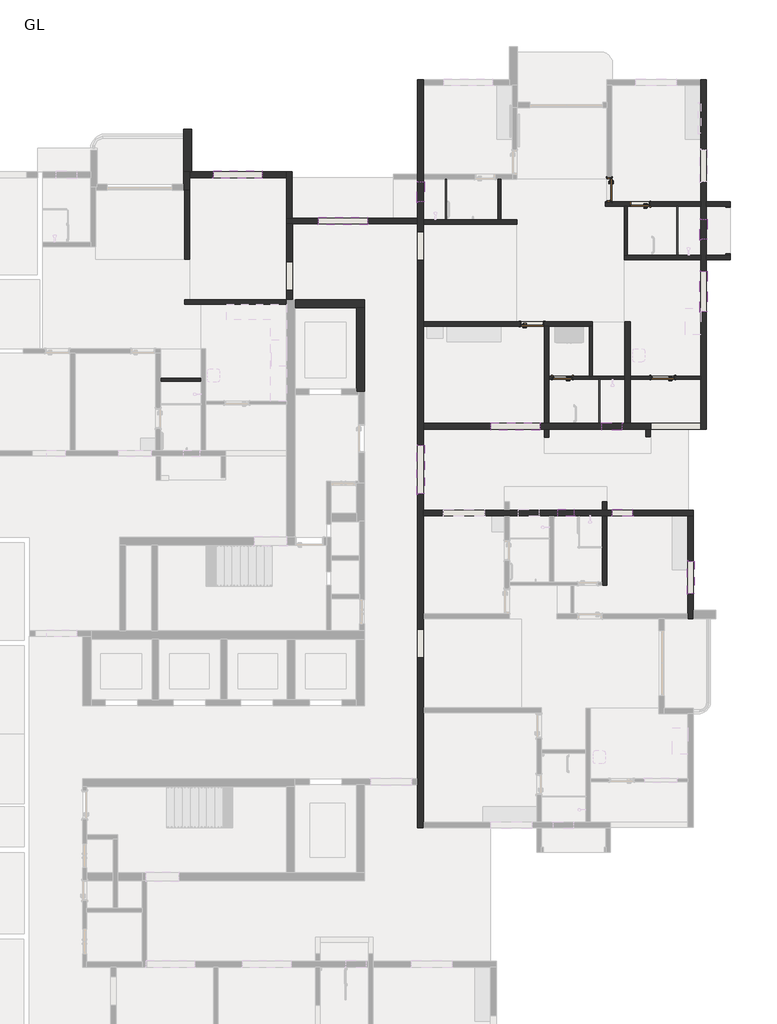
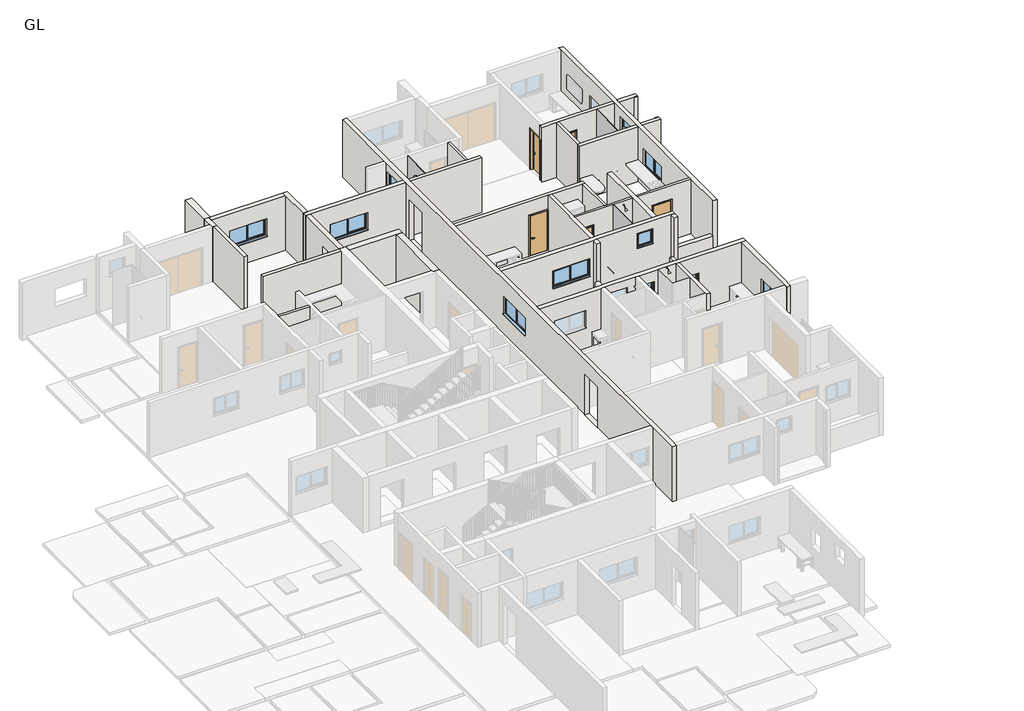
# One storey, part 6 of 14: 34 walls, 11 windows, 5 doors, 3 plates.
# Revit data of these elements (continued)
# Type "Windows_Sgl_Plain : 2'" (continued)
#   Material Frame = Window Frame
#   Wall Closure = (empty or 0)
# Type "Windows_Sgl_Plain : 2.5'"
#   Type Mark = "61"
#   Operation = "SinglePanel"
#   Construction Type Id = "SGL"
#   Manufacturer = "Revit"
#   Keynote = "L10"
#   Analytic Construction = "Large single-glazed windows"
#   Wrap Layers (Ext) from Ext = 0.336286 ft
#   Wrap Layers (Int) from Ext = 0.582349 ft
#   Window Board Projection = 0.082021 ft
#   Window Board Extension = 0.082021 ft
#   Visual Light Transmittance = 0.9
#   Solar Heat Gain Coefficient = 0.86
#   Rough Width = 2.5 ft
#   Rough Height = 2.5 ft
#   Height = 2.5 ft
#   Width = 2.5 ft
#   Heat Transfer Coefficient (U) = 5.5617 W/(m²·K)
#   Glazing Thickness = 0.07874 ft
#   FrameOffset - External = 0.164042 ft
#   Frame Depth = 0.213255 ft
#   Default Head Height = 6.922572 ft
#   Cill Depth = 0.287073 ft
#   Cavity Closer Width = 0.164042 ft
#   Cavity Closer Offset from Ext = 0.336286 ft
#   Cavity Closer Depth = 0.278871 ft
#   Vis - Cavity Closers = yes
#   Define Thermal Properties by = 1
#   Material Trim = Window Frame
#   Material Glass = Glass
#   Material Frame = Window Frame
#   Wall Closure = (empty or 0)
# Elements 1, 2 (IfcDoor, "Doors_IntSgl : 2.5' DOOR")
#   Phase Created = New Construction
#   Materials on its faces: "Door - Architrave", "Door - Handle", "Door - Frame/Mullion (1)", "Door - Panel"
# Elements 3, 4, 5 (IfcDoor, "Doors_IntSgl : 3' DOOR")
#   Phase Created = New Construction
#   Materials on its faces: "Door - Architrave", "Door - Handle", "Door - Frame/Mullion (1)", "Door - Panel"
# Elements 6, 7, 8 (IfcPlate, "System Panel : Glazed")
#   Phase Created = New Construction
#   Materials on its faces: "Glass"
# Elements 9, 10, 11, 12, 13, 14, 15, 16, 17, 18, 19, 20, 21, 22 (IfcWall, "W2")
#   Top Offset = 0.0 ft
#   Base Offset = 0.0 ft
#   wall height = 9.84252 ft
#   Phase Created = New Construction
#   Base Constraint = GL
#   Top Constraint = FFL
#   Materials on its faces: "Brick, Common"
# Elements 23, 24, 25, 26, 27 (IfcWall, "W3")
#   Top Offset = 0.0 ft
#   Base Offset = 0.0 ft
#   wall height = 9.84252 ft
#   Phase Created = New Construction
#   Base Constraint = GL
#   Top Constraint = FFL
#   Materials on its faces: "Brick, Common"
# Elements 28, 29, 30 (IfcWall, "W4")
#   Top Offset = 0.0 ft
#   Base Offset = 0.0 ft
#   wall height = 9.84252 ft
#   Phase Created = New Construction
#   Base Constraint = GL
#   Top Constraint = FFL
#   Materials on its faces: "Brick, Common"
# Element 31 (IfcWall, "W7")
#   Top Offset = 0.0 ft
#   Base Offset = 0.0 ft
#   wall height = 9.84252 ft
#   Phase Created = New Construction
#   Base Constraint = GL
#   Top Constraint = FFL
#   Materials on its faces: "Brick, Common"
# Elements 32, 33, 34, 35, 36, 37, 39, 40, 41, 42 (IfcWall, "W8")
#   Top Offset = 0.0 ft
#   Base Offset = 0.0 ft
#   wall height = 9.84252 ft
#   Phase Created = New Construction
#   Base Constraint = GL
#   Top Constraint = FFL
#   Materials on its faces: "Brick, Common"
# Element 38 (IfcWall, "W8")
#   Top Offset = -6.0 ft
#   Base Offset = 0.0 ft
#   wall height = 3.84252 ft
#   Phase Created = New Construction
#   Base Constraint = GL
#   Top Constraint = FFL
#   Materials on its faces: "Brick, Common"
# Element 43 (IfcWindow, "Windows_Dbl_Plain : 2.5'")
#   Mark = "32"
#   Phase Created = New Construction
#   Materials on its faces: "Window Frame", "Glass"
# Element 44 (IfcWindow, "Windows_Dbl_Plain : 4'")
#   Mark = "31"
#   Phase Created = New Construction
#   Materials on its faces: "Window Frame", "Glass"
# Element 45 (IfcWindow, "Windows_Dbl_Plain : 5'")
#   Mark = "39"
#   Phase Created = New Construction
#   Materials on its faces: "Window Frame", "Glass"
# Element 46 (IfcWindow, "Windows_Dbl_Plain : 6'")
#   Mark = "36"
#   Phase Created = New Construction
#   Materials on its faces: "Window Frame", "Glass"
# Element 47 (IfcWindow, "Windows_Dbl_Plain : 6'")
#   Mark = "37"
#   Phase Created = New Construction
#   Materials on its faces: "Window Frame", "Glass"
# Element 48 (IfcWindow, "Windows_Dbl_Plain : 6'")
#   Mark = "46"
#   Phase Created = New Construction
#   Materials on its faces: "Window Frame", "Glass"
# Element 49 (IfcWindow, "Windows_Dbl_Plain : 6'")
#   Mark = "47"
#   Phase Created = New Construction
#   Materials on its faces: "Window Frame", "Glass"
# Element 50 (IfcWindow, "Windows_Sgl_Plain : 2'")
#   Mark = "33"
#   Phase Created = New Construction
#   Materials on its faces: "Window Frame", "Glass"
# Element 51 (IfcWindow, "Windows_Sgl_Plain : 2.5'")
#   Mark = "38"
#   Phase Created = New Construction
#   Materials on its faces: "Window Frame", "Glass"
# Element 52 (IfcWindow, "Windows_Sgl_Plain : 2.5'")
#   Mark = "40"
#   Phase Created = New Construction
#   Materials on its faces: "Window Frame", "Glass"
# Element 53 (IfcWindow, "Windows_Sgl_Plain : 2.5'")
#   Mark = "45"
#   Phase Created = New Construction
#   Materials on its faces: "Window Frame", "Glass"
# Materials
#   "Door - Handle": colour RGB 0 0 0, transparency 0, Keynote = "P21", Cost = 0
#   "Door - Frame/Mullion (1)": class "Wood", colour RGB 212 179 113, transparency 0, Keynote = "L20", Cost = 0
#   "Door - Panel": class "Wood", colour RGB 210 159 95, transparency 0, Keynote = "L20", Cost = 0
#   "Door - Architrave": class "Wood", colour RGB 154 90 5, transparency 0, Keynote = "P20", Cost = 0
#   "Brick, Common": class "Masonry", colour RGB 170 100 105, transparency 0, Description = "Common brick", Cost = 0
#   "Window Frame": colour RGB 249 249 249, transparency 0, Keynote = "L10", Cost = 0
#   "Glass": class "Glass", colour RGB 0 128 192, transparency 0.9, Description = "Soda Lime Glass", Cost = 0
